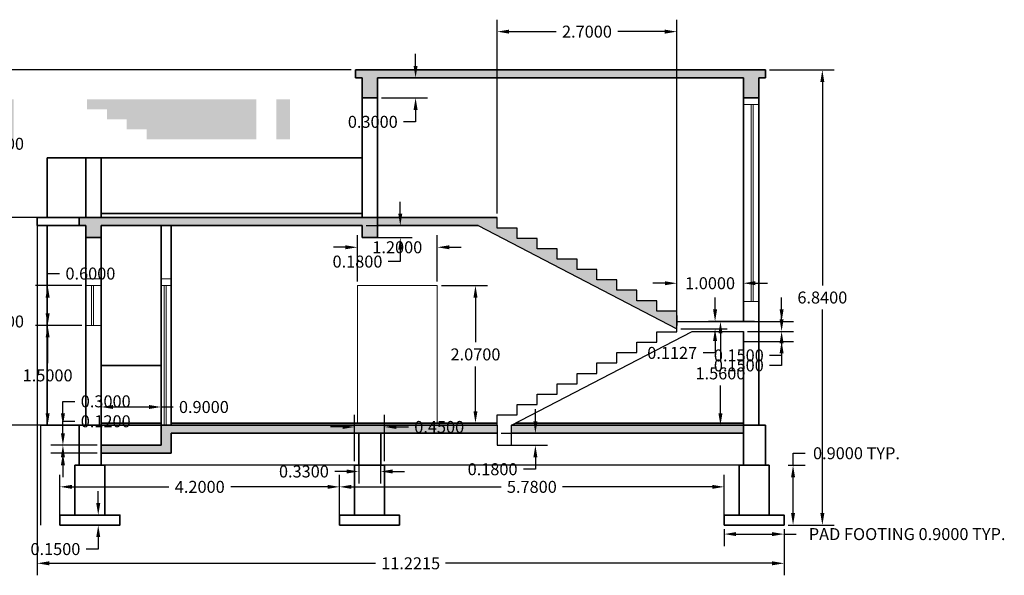
# Model space of a CAD drawing. Units: metres. Extents: x 5.2 to 41.7, y 12.2 to 37.4.
# Tile 6 of 6: x 26.9 to 41.7, y 28.3 to 36.7. Entities that reach past the tile are written whole.
import ezdxf

# ---------------------------------------------------------------- set-up
doc = ezdxf.new("R2010")
doc.units = ezdxf.units.M
doc.header["$MEASUREMENT"] = 0
for name, color, linetype, lineweight in [('A-ANNO-DIMS', 2, 'Continuous', 18), ('A-DOOR', 4, 'Continuous', 18), ('A-FLOR-PLIN', 7, 'Continuous', 25), ('A-FLOR-STRS', 7, 'Continuous', 25), ('A-SECT', 7, 'Continuous', 35), ('S-FNDN', 1, 'Continuous', 35), ('S-SLAB', 7, 'Continuous', 35)]:
    doc.layers.add(name, color=color, linetype=linetype, lineweight=lineweight)
for name, color, linetype, lineweight, true_color in [('A-GLAZ', 51, 'Continuous', 18, 0xf7f281), ('A-PLIN-PATT', 251, 'Continuous', 13, 0x636466), ('S-CONC-PATT', 251, 'Continuous', 13, 0x636466)]:
    doc.layers.add(name, color=color, linetype=linetype, lineweight=lineweight, true_color=true_color)
doc.styles.get("Standard").update_dxf_attribs({"font": 'arial.ttf'})
doc.dimstyles.get("Standard").update_dxf_attribs({"dimtxt": 0.18, "dimasz": 0.18, "dimexe": 0.18, "dimexo": 0.0625, "dimgap": 0.09, "dimtad": 0, "dimtih": 1, "dimtoh": 1, "dimdec": 4, "dimzin": 0, "dimdsep": 46, "dimtxsty": 'Standard', "dimcen": 0.09, "dimadec": 0, "dimazin": 0, "dimtfac": 1, "dimtdec": 4, "dimtofl": 0, "dimtmove": 0, "dimatfit": 3, "dimfxl": 1, "dimtolj": 1, "dimtzin": 0, "dimarcsym": 0})

# ---------------------------------------------------------------- blocks, each defined once
blk = doc.blocks.new('PAD-FOOTING-SECT-900')
for points in [[(0.225, 0.9), (0.675, 0.9), (0.675, 0.15), (0.225, 0.15)], [(0, 0.15), (0.9, 0.15), (0.9, 0), (0, 0)]]:
    blk.add_lwpolyline(points, close=True)
blk = doc.blocks.new('*D24')
at = {"layer": 'A-ANNO-DIMS', "color": 0, "lineweight": -2, "transparency": 16777216}
for p, q in [((37.489, 29.018), (37.489, 28.765)), ((38.389, 29.018), (38.389, 28.765)), ((37.669, 28.945), (38.209, 28.945)), ((38.389, 28.945), (38.569, 28.945))]:
    blk.add_line(p, q, dxfattribs=at)
at = {"layer": 'A-ANNO-DIMS', "color": 0, "lineweight": 25, "transparency": 16777216}
for points in [[(37.669, 28.975), (37.669, 28.915), (37.489, 28.945)], [(38.209, 28.975), (38.209, 28.915), (38.389, 28.945)]]:
    blk.add_solid(points, dxfattribs=at)
at = {"layer": 'Defpoints', "color": 0, "lineweight": 25, "transparency": 16777216}
for p in [(37.489, 29.08), (38.389, 29.08), (38.389, 28.945)]:
    blk.add_point(p, dxfattribs=at)
at = {"layer": 'A-ANNO-DIMS', "color": 0, "transparency": 16777216, "insert": (40.238, 28.945), "char_height": 0.18, "attachment_point": 5}
blk.add_mtext('\\A1;PAD FOOTING 0.9000 TYP.', dxfattribs=at)
blk = doc.blocks.new('*D25')
at = {"layer": 'A-ANNO-DIMS', "color": 0, "lineweight": -2, "transparency": 16777216}
for p, q in [((38.524, 29.98), (38.524, 30.16)), ((38.524, 30.16), (38.704, 30.16)), ((38.452, 29.98), (38.704, 29.98)), ((38.524, 29.26), (38.524, 29.8)), ((38.452, 29.08), (38.704, 29.08))]:
    blk.add_line(p, q, dxfattribs=at)
at = {"layer": 'A-ANNO-DIMS', "color": 0, "lineweight": 25, "transparency": 16777216}
for points in [[(38.494, 29.8), (38.554, 29.8), (38.524, 29.98)], [(38.494, 29.26), (38.554, 29.26), (38.524, 29.08)]]:
    blk.add_solid(points, dxfattribs=at)
at = {"layer": 'Defpoints', "color": 0, "lineweight": 25, "transparency": 16777216}
for p in [(38.389, 29.98), (38.524, 29.98), (38.389, 29.08)]:
    blk.add_point(p, dxfattribs=at)
at = {"layer": 'A-ANNO-DIMS', "color": 0, "transparency": 16777216, "insert": (39.477, 30.16), "char_height": 0.18, "attachment_point": 5}
blk.add_mtext('\\A1;0.9000 TYP.', dxfattribs=at)
blk = doc.blocks.new('*D46')
at = {"layer": 'A-ANNO-DIMS', "color": 0, "lineweight": -2, "transparency": 16777216}
for p, q in [((27.167, 33.638), (27.167, 28.326)), ((38.389, 29.018), (38.389, 28.326)), ((27.347, 28.506), (32.252, 28.506)), ((38.209, 28.506), (33.304, 28.506))]:
    blk.add_line(p, q, dxfattribs=at)
at = {"layer": 'A-ANNO-DIMS', "color": 0, "lineweight": 25, "transparency": 16777216}
for points in [[(27.347, 28.536), (27.347, 28.476), (27.167, 28.506)], [(38.209, 28.536), (38.209, 28.476), (38.389, 28.506)]]:
    blk.add_solid(points, dxfattribs=at)
at = {"layer": 'Defpoints', "color": 0, "lineweight": 25, "transparency": 16777216}
for p in [(27.167, 33.7), (38.389, 29.08), (38.389, 28.506)]:
    blk.add_point(p, dxfattribs=at)
at = {"layer": 'A-ANNO-DIMS', "color": 0, "transparency": 16777216, "insert": (32.778, 28.506), "char_height": 0.18, "attachment_point": 5}
blk.add_mtext('\\A1;11.2215', dxfattribs=at)
blk = doc.blocks.new('*D47')
at = {"layer": 'A-ANNO-DIMS', "color": 0, "lineweight": -2, "transparency": 16777216}
for p, q in [((38.17, 35.92), (39.144, 35.92)), ((38.964, 35.74), (38.964, 32.682)), ((38.964, 29.26), (38.964, 32.318)), ((38.452, 29.08), (39.144, 29.08))]:
    blk.add_line(p, q, dxfattribs=at)
at = {"layer": 'A-ANNO-DIMS', "color": 0, "lineweight": 25, "transparency": 16777216}
for points in [[(38.934, 35.74), (38.994, 35.74), (38.964, 35.92)], [(38.934, 29.26), (38.994, 29.26), (38.964, 29.08)]]:
    blk.add_solid(points, dxfattribs=at)
at = {"layer": 'Defpoints', "color": 0, "lineweight": 25, "transparency": 16777216}
for p in [(38.107, 35.92), (38.964, 35.92), (38.389, 29.08)]:
    blk.add_point(p, dxfattribs=at)
at = {"layer": 'A-ANNO-DIMS', "color": 0, "transparency": 16777216, "insert": (38.964, 32.5), "char_height": 0.18, "attachment_point": 5}
blk.add_mtext('\\A1;6.8400', dxfattribs=at)
blk = doc.blocks.new('*D48')
at = {"layer": 'A-ANNO-DIMS', "color": 0, "lineweight": -2, "transparency": 16777216}
for p, q in [((27.509, 29.143), (27.509, 29.835)), ((31.709, 29.143), (31.709, 29.835)), ((27.689, 29.655), (29.142, 29.655)), ((31.529, 29.655), (30.076, 29.655))]:
    blk.add_line(p, q, dxfattribs=at)
at = {"layer": 'A-ANNO-DIMS', "color": 0, "lineweight": 25, "transparency": 16777216}
for points in [[(27.689, 29.685), (27.689, 29.625), (27.509, 29.655)], [(31.529, 29.685), (31.529, 29.625), (31.709, 29.655)]]:
    blk.add_solid(points, dxfattribs=at)
at = {"layer": 'Defpoints', "color": 0, "lineweight": 25, "transparency": 16777216}
for p in [(31.709, 29.655), (27.509, 29.08), (31.709, 29.08)]:
    blk.add_point(p, dxfattribs=at)
at = {"layer": 'A-ANNO-DIMS', "color": 0, "transparency": 16777216, "insert": (29.609, 29.655), "char_height": 0.18, "attachment_point": 5}
blk.add_mtext('\\A1;4.2000', dxfattribs=at)
blk = doc.blocks.new('*D49')
at = {"layer": 'A-ANNO-DIMS', "color": 0, "lineweight": -2, "transparency": 16777216}
for p, q in [((31.709, 29.143), (31.709, 29.835)), ((37.489, 29.143), (37.489, 29.835)), ((31.889, 29.655), (34.136, 29.655)), ((37.309, 29.655), (35.062, 29.655))]:
    blk.add_line(p, q, dxfattribs=at)
at = {"layer": 'A-ANNO-DIMS', "color": 0, "lineweight": 25, "transparency": 16777216}
for points in [[(31.889, 29.685), (31.889, 29.625), (31.709, 29.655)], [(37.309, 29.685), (37.309, 29.625), (37.489, 29.655)]]:
    blk.add_solid(points, dxfattribs=at)
at = {"layer": 'Defpoints', "color": 0, "lineweight": 25, "transparency": 16777216}
for p in [(37.489, 29.655), (31.709, 29.08), (37.489, 29.08)]:
    blk.add_point(p, dxfattribs=at)
at = {"layer": 'A-ANNO-DIMS', "color": 0, "transparency": 16777216, "insert": (34.599, 29.655), "char_height": 0.18, "attachment_point": 5}
blk.add_mtext('\\A1;5.7800', dxfattribs=at)
blk = doc.blocks.new('*D50')
at = {"layer": 'A-ANNO-DIMS', "color": 0, "lineweight": -2, "transparency": 16777216}
for p, q in [((28.065, 33.7), (26.413, 33.7)), ((26.593, 33.52), (26.593, 32.322)), ((26.593, 30.76), (26.593, 31.958)), ((28.065, 30.58), (26.413, 30.58))]:
    blk.add_line(p, q, dxfattribs=at)
at = {"layer": 'A-ANNO-DIMS', "color": 0, "lineweight": 25, "transparency": 16777216}
for points in [[(26.563, 33.52), (26.623, 33.52), (26.593, 33.7)], [(26.563, 30.76), (26.623, 30.76), (26.593, 30.58)]]:
    blk.add_solid(points, dxfattribs=at)
at = {"layer": 'Defpoints', "color": 0, "lineweight": 25, "transparency": 16777216}
for p in [(26.593, 33.7), (28.127, 33.7), (28.127, 30.58)]:
    blk.add_point(p, dxfattribs=at)
at = {"layer": 'A-ANNO-DIMS', "color": 0, "transparency": 16777216, "insert": (26.593, 32.14), "char_height": 0.18, "attachment_point": 5}
blk.add_mtext('\\A1;3.1200', dxfattribs=at)
blk = doc.blocks.new('*D51')
at = {"layer": 'A-ANNO-DIMS', "color": 0, "lineweight": -2, "transparency": 16777216}
for p, q in [((37.945, 32.14), (37.253, 32.14)), ((37.433, 31.96), (37.433, 31.542)), ((37.433, 30.76), (37.433, 31.178)), ((37.945, 30.58), (37.253, 30.58))]:
    blk.add_line(p, q, dxfattribs=at)
at = {"layer": 'A-ANNO-DIMS', "color": 0, "lineweight": 25, "transparency": 16777216}
for points in [[(37.403, 31.96), (37.463, 31.96), (37.433, 32.14)], [(37.403, 30.76), (37.463, 30.76), (37.433, 30.58)]]:
    blk.add_solid(points, dxfattribs=at)
at = {"layer": 'Defpoints', "color": 0, "lineweight": 25, "transparency": 16777216}
for p in [(37.433, 32.14), (38.007, 32.14), (38.007, 30.58)]:
    blk.add_point(p, dxfattribs=at)
at = {"layer": 'A-ANNO-DIMS', "color": 0, "transparency": 16777216, "insert": (37.433, 31.36), "char_height": 0.18, "attachment_point": 5}
blk.add_mtext('\\A1;1.5600', dxfattribs=at)
blk = doc.blocks.new('*D52')
at = {"layer": 'A-ANNO-DIMS', "color": 0, "lineweight": -2, "transparency": 16777216}
for p, q in [((36.777476, 32.202757), (36.777476, 32.894757)), ((37.777476, 32.202757), (37.777476, 32.894757)), ((36.597476, 32.714757), (36.417476, 32.714757)), ((37.957476, 32.714757), (38.137476, 32.714757))]:
    blk.add_line(p, q, dxfattribs=at)
at = {"layer": 'A-ANNO-DIMS', "color": 0, "lineweight": 25, "transparency": 16777216}
for points in [[(36.597476, 32.744757), (36.597476, 32.684757), (36.777476, 32.714757)], [(37.957476, 32.744757), (37.957476, 32.684757), (37.777476, 32.714757)]]:
    blk.add_solid(points, dxfattribs=at)
at = {"layer": 'Defpoints', "color": 0, "lineweight": 25, "transparency": 16777216}
for p in [(37.777476, 32.714757), (36.777476, 32.140257), (37.777476, 32.140257)]:
    blk.add_point(p, dxfattribs=at)
at = {"layer": 'A-ANNO-DIMS', "color": 0, "transparency": 16777216, "insert": (37.277476, 32.714757), "char_height": 0.18, "attachment_point": 5}
blk.add_mtext('\\A1;1.0000', dxfattribs=at)
blk = doc.blocks.new('*D53')
at = {"layer": 'A-ANNO-DIMS', "color": 0, "lineweight": -2, "transparency": 16777216}
for p, q in [((34.077, 33.763), (34.077, 36.675)), ((36.777, 32.203), (36.777, 36.675)), ((34.257, 36.495), (34.963, 36.495)), ((36.597, 36.495), (35.892, 36.495))]:
    blk.add_line(p, q, dxfattribs=at)
at = {"layer": 'A-ANNO-DIMS', "color": 0, "lineweight": 25, "transparency": 16777216}
for points in [[(34.257, 36.525), (34.257, 36.465), (34.077, 36.495)], [(36.597, 36.525), (36.597, 36.465), (36.777, 36.495)]]:
    blk.add_solid(points, dxfattribs=at)
at = {"layer": 'Defpoints', "color": 0, "lineweight": 25, "transparency": 16777216}
for p in [(36.777, 36.495), (34.077, 33.7), (36.777, 32.14)]:
    blk.add_point(p, dxfattribs=at)
at = {"layer": 'A-ANNO-DIMS', "color": 0, "transparency": 16777216, "insert": (35.427, 36.495), "char_height": 0.18, "attachment_point": 5}
blk.add_mtext('\\A1;2.7000', dxfattribs=at)
blk = doc.blocks.new('*D54')
at = {"layer": 'A-ANNO-DIMS', "color": 0, "lineweight": -2, "transparency": 16777216}
for p, q in [((31.977476, 32.742757), (31.977476, 33.434757)), ((33.177476, 32.742757), (33.177476, 33.434757)), ((31.797476, 33.254757), (31.617476, 33.254757)), ((33.357476, 33.254757), (33.537476, 33.254757))]:
    blk.add_line(p, q, dxfattribs=at)
at = {"layer": 'A-ANNO-DIMS', "color": 0, "lineweight": 25, "transparency": 16777216}
for points in [[(31.797476, 33.284757), (31.797476, 33.224757), (31.977476, 33.254757)], [(33.357476, 33.284757), (33.357476, 33.224757), (33.177476, 33.254757)]]:
    blk.add_solid(points, dxfattribs=at)
at = {"layer": 'Defpoints', "color": 0, "lineweight": 25, "transparency": 16777216}
for p in [(33.177476, 33.254757), (31.977476, 32.680257), (33.177476, 32.680257)]:
    blk.add_point(p, dxfattribs=at)
at = {"layer": 'A-ANNO-DIMS', "color": 0, "transparency": 16777216, "insert": (32.577476, 33.254757), "char_height": 0.18, "attachment_point": 5}
blk.add_mtext('\\A1;1.2000', dxfattribs=at)
blk = doc.blocks.new('*D55')
at = {"layer": 'A-ANNO-DIMS', "color": 0, "lineweight": -2, "transparency": 16777216}
for p, q in [((33.24, 32.68), (33.932, 32.68)), ((33.752, 32.5), (33.752, 31.827)), ((33.752, 30.79), (33.752, 31.463)), ((33.24, 30.61), (33.932, 30.61))]:
    blk.add_line(p, q, dxfattribs=at)
at = {"layer": 'A-ANNO-DIMS', "color": 0, "lineweight": 25, "transparency": 16777216}
for points in [[(33.722, 32.5), (33.782, 32.5), (33.752, 32.68)], [(33.722, 30.79), (33.782, 30.79), (33.752, 30.61)]]:
    blk.add_solid(points, dxfattribs=at)
at = {"layer": 'Defpoints', "color": 0, "lineweight": 25, "transparency": 16777216}
for p in [(33.177, 32.68), (33.177, 30.61), (33.752, 30.61)]:
    blk.add_point(p, dxfattribs=at)
at = {"layer": 'A-ANNO-DIMS', "color": 0, "transparency": 16777216, "insert": (33.752, 31.645), "char_height": 0.18, "attachment_point": 5}
blk.add_mtext('\\A1;2.0700', dxfattribs=at)
blk = doc.blocks.new('*D56')
at = {"layer": 'A-ANNO-DIMS', "color": 0, "lineweight": -2, "transparency": 16777216}
for p, q in [((31.885, 35.92), (26.413, 35.92)), ((26.593, 35.74), (26.593, 34.992)), ((26.593, 33.88), (26.593, 34.628)), ((31.985, 33.7), (26.413, 33.7))]:
    blk.add_line(p, q, dxfattribs=at)
at = {"layer": 'A-ANNO-DIMS', "color": 0, "lineweight": 25, "transparency": 16777216}
for points in [[(26.563, 35.74), (26.623, 35.74), (26.593, 35.92)], [(26.563, 33.88), (26.623, 33.88), (26.593, 33.7)]]:
    blk.add_solid(points, dxfattribs=at)
at = {"layer": 'Defpoints', "color": 0, "lineweight": 25, "transparency": 16777216}
for p in [(26.593, 35.92), (31.947, 35.92), (32.047, 33.7)]:
    blk.add_point(p, dxfattribs=at)
at = {"layer": 'A-ANNO-DIMS', "color": 0, "transparency": 16777216, "insert": (26.593, 34.81), "char_height": 0.18, "attachment_point": 5}
blk.add_mtext('\\A1;2.2200', dxfattribs=at)
blk = doc.blocks.new('*D78')
at = {"layer": 'A-ANNO-DIMS', "color": 0, "lineweight": -2, "transparency": 16777216}
for p, q in [((27.835, 32.08), (27.143, 32.08)), ((27.323, 31.9), (27.323, 31.512)), ((27.323, 30.76), (27.323, 31.148)), ((27.835, 30.58), (27.143, 30.58))]:
    blk.add_line(p, q, dxfattribs=at)
at = {"layer": 'A-ANNO-DIMS', "color": 0, "lineweight": 25, "transparency": 16777216}
for points in [[(27.293, 31.9), (27.353, 31.9), (27.323, 32.08)], [(27.293, 30.76), (27.353, 30.76), (27.323, 30.58)]]:
    blk.add_solid(points, dxfattribs=at)
at = {"layer": 'Defpoints', "color": 0, "lineweight": 25, "transparency": 16777216}
for p in [(27.323, 32.08), (27.897, 32.08), (27.897, 30.58)]:
    blk.add_point(p, dxfattribs=at)
at = {"layer": 'A-ANNO-DIMS', "color": 0, "transparency": 16777216, "insert": (27.323, 31.33), "char_height": 0.18, "attachment_point": 5}
blk.add_mtext('\\A1;1.5000', dxfattribs=at)
blk = doc.blocks.new('*D79')
at = {"layer": 'A-ANNO-DIMS', "color": 0, "lineweight": -2, "transparency": 16777216}
for p, q in [((27.323, 32.68), (27.323, 32.86)), ((27.323, 32.86), (27.503, 32.86)), ((27.835, 32.68), (27.143, 32.68)), ((27.323, 32.26), (27.323, 32.5)), ((27.835, 32.08), (27.143, 32.08))]:
    blk.add_line(p, q, dxfattribs=at)
at = {"layer": 'A-ANNO-DIMS', "color": 0, "lineweight": 25, "transparency": 16777216}
for points in [[(27.293, 32.5), (27.353, 32.5), (27.323, 32.68)], [(27.293, 32.26), (27.353, 32.26), (27.323, 32.08)]]:
    blk.add_solid(points, dxfattribs=at)
at = {"layer": 'Defpoints', "color": 0, "lineweight": 25, "transparency": 16777216}
for p in [(27.323, 32.68), (27.897, 32.68), (27.897, 32.08)]:
    blk.add_point(p, dxfattribs=at)
at = {"layer": 'A-ANNO-DIMS', "color": 0, "transparency": 16777216, "insert": (27.966, 32.86), "char_height": 0.18, "attachment_point": 5}
blk.add_mtext('\\A1;0.6000', dxfattribs=at)
blk = doc.blocks.new('*D80')
at = {"layer": 'A-ANNO-DIMS', "color": 0, "lineweight": -2, "transparency": 16777216}
for p, q in [((28.084, 29.41), (28.084, 29.59)), ((27.572, 29.23), (28.264, 29.23)), ((27.572, 29.08), (28.264, 29.08)), ((28.084, 28.9), (28.084, 28.72)), ((28.084, 28.72), (27.904, 28.72))]:
    blk.add_line(p, q, dxfattribs=at)
at = {"layer": 'A-ANNO-DIMS', "color": 0, "lineweight": 25, "transparency": 16777216}
for points in [[(28.054, 29.41), (28.114, 29.41), (28.084, 29.23)], [(28.054, 28.9), (28.114, 28.9), (28.084, 29.08)]]:
    blk.add_solid(points, dxfattribs=at)
at = {"layer": 'Defpoints', "color": 0, "lineweight": 25, "transparency": 16777216}
for p in [(27.509, 29.23), (27.509, 29.08), (28.084, 29.08)]:
    blk.add_point(p, dxfattribs=at)
at = {"layer": 'A-ANNO-DIMS', "color": 0, "transparency": 16777216, "insert": (27.44, 28.72), "char_height": 0.18, "attachment_point": 5}
blk.add_mtext('\\A1;0.1500', dxfattribs=at)
blk = doc.blocks.new('*D81')
at = {"layer": 'A-ANNO-DIMS', "color": 0, "lineweight": -2, "transparency": 16777216}
for p, q in [((31.934, 30.043), (31.934, 30.735)), ((32.384, 30.043), (32.384, 30.735)), ((31.754, 30.555), (31.574, 30.555)), ((32.564, 30.555), (32.744, 30.555))]:
    blk.add_line(p, q, dxfattribs=at)
at = {"layer": 'A-ANNO-DIMS', "color": 0, "lineweight": 25, "transparency": 16777216}
for points in [[(31.754, 30.585), (31.754, 30.525), (31.934, 30.555)], [(32.564, 30.585), (32.564, 30.525), (32.384, 30.555)]]:
    blk.add_solid(points, dxfattribs=at)
at = {"layer": 'Defpoints', "color": 0, "lineweight": 25, "transparency": 16777216}
for p in [(32.384, 30.555), (31.934, 29.98), (32.384, 29.98)]:
    blk.add_point(p, dxfattribs=at)
at = {"layer": 'A-ANNO-DIMS', "color": 0, "transparency": 16777216, "insert": (33.207, 30.555), "char_height": 0.18, "attachment_point": 5}
blk.add_mtext('\\A1;0.4500', dxfattribs=at)
blk = doc.blocks.new('*D82')
at = {"layer": 'A-ANNO-DIMS', "color": 0, "lineweight": -2, "transparency": 16777216}
for p, q in [((31.997, 30.398), (31.997, 29.706)), ((32.327, 30.398), (32.327, 29.706)), ((31.817, 29.886), (31.637, 29.886)), ((32.507, 29.886), (32.687, 29.886))]:
    blk.add_line(p, q, dxfattribs=at)
at = {"layer": 'A-ANNO-DIMS', "color": 0, "lineweight": 25, "transparency": 16777216}
for points in [[(31.817, 29.916), (31.817, 29.856), (31.997, 29.886)], [(32.507, 29.916), (32.507, 29.856), (32.327, 29.886)]]:
    blk.add_solid(points, dxfattribs=at)
at = {"layer": 'Defpoints', "color": 0, "lineweight": 25, "transparency": 16777216}
for p in [(31.997, 30.46), (32.327, 30.46), (31.997, 29.886)]:
    blk.add_point(p, dxfattribs=at)
at = {"layer": 'A-ANNO-DIMS', "color": 0, "transparency": 16777216, "insert": (31.174, 29.886), "char_height": 0.18, "attachment_point": 5}
blk.add_mtext('\\A1;0.3300', dxfattribs=at)
blk = doc.blocks.new('*D83')
at = {"layer": 'A-ANNO-DIMS', "color": 0, "lineweight": -2, "transparency": 16777216}
for p, q in [((28.127, 30.343), (28.127, 31.035)), ((29.027, 30.343), (29.027, 31.035)), ((28.307, 30.855), (28.847, 30.855)), ((29.027, 30.855), (29.207, 30.855))]:
    blk.add_line(p, q, dxfattribs=at)
at = {"layer": 'A-ANNO-DIMS', "color": 0, "lineweight": 25, "transparency": 16777216}
for points in [[(28.307, 30.885), (28.307, 30.825), (28.127, 30.855)], [(28.847, 30.885), (28.847, 30.825), (29.027, 30.855)]]:
    blk.add_solid(points, dxfattribs=at)
at = {"layer": 'Defpoints', "color": 0, "lineweight": 25, "transparency": 16777216}
for p in [(29.027, 30.855), (28.127, 30.28), (29.027, 30.28)]:
    blk.add_point(p, dxfattribs=at)
at = {"layer": 'A-ANNO-DIMS', "color": 0, "transparency": 16777216, "insert": (29.671, 30.855), "char_height": 0.18, "attachment_point": 5}
blk.add_mtext('\\A1;0.9000', dxfattribs=at)
blk = doc.blocks.new('*D84')
at = {"layer": 'A-ANNO-DIMS', "color": 0, "lineweight": -2, "transparency": 16777216}
for p, q in [((27.553, 30.76), (27.553, 30.94)), ((27.553, 30.94), (27.733, 30.94)), ((28.065, 30.58), (27.373, 30.58)), ((28.065, 30.28), (27.373, 30.28)), ((27.553, 30.1), (27.553, 29.92))]:
    blk.add_line(p, q, dxfattribs=at)
at = {"layer": 'A-ANNO-DIMS', "color": 0, "lineweight": 25, "transparency": 16777216}
for points in [[(27.523, 30.76), (27.583, 30.76), (27.553, 30.58)], [(27.523, 30.1), (27.583, 30.1), (27.553, 30.28)]]:
    blk.add_solid(points, dxfattribs=at)
at = {"layer": 'Defpoints', "color": 0, "lineweight": 25, "transparency": 16777216}
for p in [(27.553, 30.58), (28.127, 30.58), (28.127, 30.28)]:
    blk.add_point(p, dxfattribs=at)
at = {"layer": 'A-ANNO-DIMS', "color": 0, "transparency": 16777216, "insert": (28.196, 30.94), "char_height": 0.18, "attachment_point": 5}
blk.add_mtext('\\A1;0.3000', dxfattribs=at)
blk = doc.blocks.new('*D85')
at = {"layer": 'A-ANNO-DIMS', "color": 0, "lineweight": -2, "transparency": 16777216}
for p, q in [((27.553, 30.46), (27.553, 30.64)), ((27.553, 30.64), (27.733, 30.64)), ((28.065, 30.28), (27.373, 30.28)), ((28.065, 30.16), (27.373, 30.16)), ((27.553, 29.98), (27.553, 29.8))]:
    blk.add_line(p, q, dxfattribs=at)
at = {"layer": 'A-ANNO-DIMS', "color": 0, "lineweight": 25, "transparency": 16777216}
for points in [[(27.523, 30.46), (27.583, 30.46), (27.553, 30.28)], [(27.523, 29.98), (27.583, 29.98), (27.553, 30.16)]]:
    blk.add_solid(points, dxfattribs=at)
at = {"layer": 'Defpoints', "color": 0, "lineweight": 25, "transparency": 16777216}
for p in [(27.553, 30.28), (28.127, 30.28), (28.127, 30.16)]:
    blk.add_point(p, dxfattribs=at)
at = {"layer": 'A-ANNO-DIMS', "color": 0, "transparency": 16777216, "insert": (28.196, 30.64), "char_height": 0.18, "attachment_point": 5}
blk.add_mtext('\\A1;0.1200', dxfattribs=at)
blk = doc.blocks.new('*D86')
at = {"layer": 'A-ANNO-DIMS', "color": 0, "lineweight": -2, "transparency": 16777216}
for p, q in [((32.622, 33.76), (32.622, 33.94)), ((32.11, 33.58), (32.802, 33.58)), ((32.11, 33.4), (32.802, 33.4)), ((32.622, 33.22), (32.622, 33.04)), ((32.622, 33.04), (32.442, 33.04))]:
    blk.add_line(p, q, dxfattribs=at)
at = {"layer": 'A-ANNO-DIMS', "color": 0, "lineweight": 25, "transparency": 16777216}
for points in [[(32.592, 33.76), (32.652, 33.76), (32.622, 33.58)], [(32.592, 33.22), (32.652, 33.22), (32.622, 33.4)]]:
    blk.add_solid(points, dxfattribs=at)
at = {"layer": 'Defpoints', "color": 0, "lineweight": 25, "transparency": 16777216}
for p in [(32.047, 33.58), (32.047, 33.4), (32.622, 33.4)]:
    blk.add_point(p, dxfattribs=at)
at = {"layer": 'A-ANNO-DIMS', "color": 0, "transparency": 16777216, "insert": (31.979, 33.04), "char_height": 0.18, "attachment_point": 5}
blk.add_mtext('\\A1;0.1800', dxfattribs=at)
blk = doc.blocks.new('*D87')
at = {"layer": 'A-ANNO-DIMS', "color": 0, "lineweight": -2, "transparency": 16777216}
for p, q in [((32.852, 35.98), (32.852, 36.16)), ((32.34, 35.8), (33.032, 35.8)), ((32.34, 35.5), (33.032, 35.5)), ((32.852, 35.32), (32.852, 35.14)), ((32.852, 35.14), (32.672, 35.14))]:
    blk.add_line(p, q, dxfattribs=at)
at = {"layer": 'A-ANNO-DIMS', "color": 0, "lineweight": 25, "transparency": 16777216}
for points in [[(32.822, 35.98), (32.882, 35.98), (32.852, 35.8)], [(32.822, 35.32), (32.882, 35.32), (32.852, 35.5)]]:
    blk.add_solid(points, dxfattribs=at)
at = {"layer": 'Defpoints', "color": 0, "lineweight": 25, "transparency": 16777216}
for p in [(32.277, 35.8), (32.277, 35.5), (32.852, 35.5)]:
    blk.add_point(p, dxfattribs=at)
at = {"layer": 'A-ANNO-DIMS', "color": 0, "transparency": 16777216, "insert": (32.209, 35.14), "char_height": 0.18, "attachment_point": 5}
blk.add_mtext('\\A1;0.3000', dxfattribs=at)
blk = doc.blocks.new('*D88')
at = {"layer": 'A-ANNO-DIMS', "color": 0, "lineweight": -2, "transparency": 16777216}
for p, q in [((38.352, 32.17), (38.352, 32.35)), ((37.84, 31.99), (38.532, 31.99)), ((37.84, 31.84), (38.532, 31.84)), ((38.352, 31.66), (38.352, 31.48)), ((38.352, 31.48), (38.172, 31.48))]:
    blk.add_line(p, q, dxfattribs=at)
at = {"layer": 'A-ANNO-DIMS', "color": 0, "lineweight": 25, "transparency": 16777216}
for points in [[(38.322, 32.17), (38.382, 32.17), (38.352, 31.99)], [(38.322, 31.66), (38.382, 31.66), (38.352, 31.84)]]:
    blk.add_solid(points, dxfattribs=at)
at = {"layer": 'Defpoints', "color": 0, "lineweight": 25, "transparency": 16777216}
for p in [(37.777, 31.99), (37.777, 31.84), (38.352, 31.84)]:
    blk.add_point(p, dxfattribs=at)
at = {"layer": 'A-ANNO-DIMS', "color": 0, "transparency": 16777216, "insert": (37.709, 31.48), "char_height": 0.18, "attachment_point": 5}
blk.add_mtext('\\A1;0.1500', dxfattribs=at)
blk = doc.blocks.new('*D89')
at = {"layer": 'A-ANNO-DIMS', "color": 0, "lineweight": -2, "transparency": 16777216}
for p, q in [((38.352, 32.32), (38.352, 32.5)), ((37.84, 32.14), (38.532, 32.14)), ((37.84, 31.99), (38.532, 31.99)), ((38.352, 31.81), (38.352, 31.63)), ((38.352, 31.63), (38.172, 31.63))]:
    blk.add_line(p, q, dxfattribs=at)
at = {"layer": 'A-ANNO-DIMS', "color": 0, "lineweight": 25, "transparency": 16777216}
for points in [[(38.322, 32.32), (38.382, 32.32), (38.352, 32.14)], [(38.322, 31.81), (38.382, 31.81), (38.352, 31.99)]]:
    blk.add_solid(points, dxfattribs=at)
at = {"layer": 'Defpoints', "color": 0, "lineweight": 25, "transparency": 16777216}
for p in [(37.777, 32.14), (37.777, 31.99), (38.352, 31.99)]:
    blk.add_point(p, dxfattribs=at)
at = {"layer": 'A-ANNO-DIMS', "color": 0, "transparency": 16777216, "insert": (37.709, 31.63), "char_height": 0.18, "attachment_point": 5}
blk.add_mtext('\\A1;0.1500', dxfattribs=at)
blk = doc.blocks.new('*D90')
at = {"layer": 'A-ANNO-DIMS', "color": 0, "lineweight": -2, "transparency": 16777216}
for p, q in [((37.352, 32.32), (37.352, 32.5)), ((36.84, 32.14), (37.532, 32.14)), ((36.84, 32.028), (37.532, 32.028)), ((37.352, 31.848), (37.352, 31.668)), ((37.352, 31.668), (37.172, 31.668))]:
    blk.add_line(p, q, dxfattribs=at)
at = {"layer": 'A-ANNO-DIMS', "color": 0, "lineweight": 25, "transparency": 16777216}
for points in [[(37.322, 32.32), (37.382, 32.32), (37.352, 32.14)], [(37.322, 31.848), (37.382, 31.848), (37.352, 32.028)]]:
    blk.add_solid(points, dxfattribs=at)
at = {"layer": 'Defpoints', "color": 0, "lineweight": 25, "transparency": 16777216}
for p in [(36.777, 32.14), (36.777, 32.028), (37.352, 32.028)]:
    blk.add_point(p, dxfattribs=at)
at = {"layer": 'A-ANNO-DIMS', "color": 0, "transparency": 16777216, "insert": (36.708, 31.668), "char_height": 0.18, "attachment_point": 5}
blk.add_mtext('\\A1;0.1127', dxfattribs=at)
blk = doc.blocks.new('*D91')
at = {"layer": 'A-ANNO-DIMS', "color": 0, "lineweight": -2, "transparency": 16777216}
for p, q in [((34.652, 30.64), (34.652, 30.82)), ((34.14, 30.46), (34.832, 30.46)), ((34.14, 30.28), (34.832, 30.28)), ((34.652, 30.1), (34.652, 29.92)), ((34.652, 29.92), (34.472, 29.92))]:
    blk.add_line(p, q, dxfattribs=at)
at = {"layer": 'A-ANNO-DIMS', "color": 0, "lineweight": 25, "transparency": 16777216}
for points in [[(34.622, 30.64), (34.682, 30.64), (34.652, 30.46)], [(34.622, 30.1), (34.682, 30.1), (34.652, 30.28)]]:
    blk.add_solid(points, dxfattribs=at)
at = {"layer": 'Defpoints', "color": 0, "lineweight": 25, "transparency": 16777216}
for p in [(34.077, 30.46), (34.077, 30.28), (34.652, 30.28)]:
    blk.add_point(p, dxfattribs=at)
at = {"layer": 'A-ANNO-DIMS', "color": 0, "transparency": 16777216, "insert": (34.009, 29.92), "char_height": 0.18, "attachment_point": 5}
blk.add_mtext('\\A1;0.1800', dxfattribs=at)

msp = doc.modelspace()

# ---------------------------------------------------------------- hatches: boundary and pattern name
at = {"layer": 'A-PLIN-PATT'}
h = msp.add_hatch(dxfattribs=at)
h.set_pattern_fill('GRAVEL', color=256, scale=0.02)
h.set_pattern_definition([(228.0127875, (0.0144, 0.02), (-0.16, -0.18), [0.00269072, -0.266381761]), (184.9697407, (0.0126, 0.018), (0.24, 0.02), [0.00461736, -0.457118495]), (132.510447, (0.008, 0.0176), (0.2, -0.22), [0.00325576, -0.322320652]), (267.273689, (0.0002, 0.0126), (0.02, 0.4), [0.00420476, -0.416271161]), (292.8336542, (0, 0.0084), (-0.1, 0.24), [0.0041231, -0.4081874626]), (357.273689, (0.0016, 0.0046), (-0.4, 0.02), [0.00420476, -0.416271161]), (37.6942405, (0.0058, 0.0044), (-0.26, -0.2), [0.00556058, -0.550496971]), (72.2553284, (0.0102, 0.0078), (0.14, 0.44), [0.00524976, -0.51972643]), (121.4295656, (0.0118, 0.0128), (-0.16, 0.26), [0.004219, -0.417681462]), (175.2363583, (0.0096, 0.0164), (0.22, -0.02), [0.00481664, -0.2360152516]), (222.3974378, (0.0048, 0.0168), (-0.24, -0.22), [0.00622896, -0.6166675]), (138.814075, (0.02, 0.0124), (-0.14, 0.12), [0.00212602, -0.210476896]), (171.4692344, (0.0184, 0.0138), (0.26, -0.04), [0.00404474, -0.400430228]), (225, (0.0144, 0.0144), (0, -0.02), [0.00282842, -0.025455851]), (203.1985905, (0.013, 0.0168), (0.1, 0.04), [0.00152316, -0.150792302]), (291.8014095, (0.0116, 0.0162), (-0.02, 0.06), [0.00215406, -0.105549236]), (30.9637565, (0.0124, 0.0142), (0.06, 0.04), [0.00349858, -0.113120458]), (161.565051, (0.0154, 0.016), (0.04, -0.02), [0.00252982, -0.060715733]), (16.3895403, (0, 0.0162), (0.2, 0.06), [0.003544, -0.350856903]), (70.346176, (0.0034, 0.0172), (-0.08, -0.22), [0.00297322, -0.294348155]), (293.1985905, (0.0154, 0.02), (-0.04, 0.1), [0.0030463, -0.149269162]), (343.6104597, (0.0166, 0.0172), (-0.2, 0.06), [0.003544, -0.350856903]), (339.443955, (0, 0.0038), (-0.1, 0.04), [0.0034176, -0.167462475]), (294.7751406, (0.0032, 0.0026), (-0.1, 0.22), [0.00286356, -0.283492861]), (66.8014095, (0.0156, 0), (0.04, 0.1), [0.0030463, -0.149269162]), (17.3540246, (0.0168, 0.0028), (-0.26, -0.08), [0.00335262, -0.331908472]), (69.443955, (0.0058, 0), (-0.04, -0.1), [0.0017088, -0.169171275]), (101.309932, (0.0144, 0), (-0.02, 0.08), [0.0010198, -0.10096059]), (165.963757, (0.0142, 0.001), (0.06, -0.02), [0.0041231, -0.0783390125]), (186.009006, (0.0102, 0.002), (0.2, 0.02), [0.003821, -0.3782784635]), (303.690068, (0.0124, 0.0124), (-0.02, 0.04), [0.00288444, -0.0692265855]), (353.1572266, (0.014, 0.01), (0.34, -0.04), [0.00503588, -0.4985512525]), (60.945396, (0.019, 0.0094), (-0.08, -0.14), [0.00205912, -0.203853483]), (90, (0.02, 0.0112), (-0.02, 0.02), [0.0012, -0.0188]), (120.256437, (0.0098, 0.0026), (0.08, -0.14), [0.00277848, -0.2750704]), (48.0127875, (0.0084, 0.005), (0.16, 0.18), [0.00538144, -0.263691041]), (0, (0.012, 0.009), (0.02, 0.02), [0.0052, -0.0148]), (325.3048465, (0.0172, 0.009), (0.2, -0.14), [0.00316228, -0.313065486]), (254.054604, (0.0198, 0.0072), (-0.02, -0.08), [0.00291204, -0.142690158]), (207.6459754, (0.019, 0.0044), (-0.38, -0.2), [0.0047413, -0.469389484]), (175.4260787, (0.0148, 0.0022), (-0.26, 0.02), [0.00501598, -0.496581468])])
h.paths.add_polyline_path([(23.80317, 35.47718), (20.65317, 35.47718), (20.65317, 34.87718), (23.80317, 34.87718)])
h.paths.add_polyline_path([(26.81317, 35.47718), (26.71317, 35.47718), (23.80317, 35.47718), (23.80317, 34.87718), (26.81317, 34.87718)])
h.paths.add_polyline_path([(30.46113, 35.47718), (27.91317, 35.47718), (27.91317, 35.32718), (28.21317, 35.32718), (28.21317, 35.17718), (28.51317, 35.17718), (28.51317, 35.02718), (28.81317, 35.02718), (28.81317, 34.87718), (30.46113, 34.87718)])
h.paths.add_polyline_path([(30.96317, 35.47718), (30.76113, 35.47718), (30.76113, 34.87718), (30.96317, 34.87718)])
at = {"layer": 'S-CONC-PATT'}
h = msp.add_hatch(dxfattribs=at)
h.set_pattern_fill('AR-CONC', color=256, scale=0.01)
h.set_pattern_definition([(50, (-29.48366, -4.896924), (0.07172602, -0.006275213), [0.0075, -0.0825]), (355, (-29.48366, -4.896924), (-0.01387513, 0.07521921), [0.006, -0.066]), (100.45144, (-29.477686, -4.89745), (0.057850885, 0.068944), [0.00637402, -0.07011421]), (46.1842, (-29.48366, -4.876924), (0.10672413, -0.01655193), [0.01125, -0.12375]), (96.63564, (-29.47477, -4.8783), (0.0934662, 0.09741186), [0.00956103, -0.10517138]), (351.18416, (-29.48366, -4.87692), (0.0934662, 0.09741186), [0.009, -0.099]), (21, (-29.47366, -4.881924), (0.059690705, -0.04026189), [0.0075, -0.0825]), (326, (-29.47366, -4.881924), (0.02433153, 0.072515005), [0.006, -0.066]), (71.45144, (-29.46869, -4.88528), (0.08402224, 0.032253115), [0.00637402, -0.07011421]), (37.5, (-29.483663, -4.896924), (0.0012159855, 0.033289385), [0, -0.0652, 0, -0.067, 0, -0.06625]), (7.5, (-29.483663, -4.896924), (0.026306954, 0.039441171), [0, -0.0382, 0, -0.0637, 0, -0.02525]), (327.5, (-29.505963, -4.896924), (0.053382244, -0.002255487), [0, -0.025, 0, -0.078, 0, -0.1035]), (317.5, (-29.515963, -4.896924), (0.058318617, 0.010010498), [0, -0.0325, 0, -0.0518, 0, -0.0735])])
h.paths.add_polyline_path([(32.27748, 33.70026), (27.79748, 33.70026), (27.79748, 33.58026), (27.89748, 33.58026), (27.89748, 33.40026), (28.12748, 33.40026), (28.12748, 33.58026), (32.04748, 33.58026), (32.04748, 33.40026), (32.27748, 33.40026)])
h.paths.add_polyline_path([(29.17748, 30.46026), (34.07748, 30.46026), (34.07748, 30.58026), (29.02748, 30.58026), (29.02748, 30.28026), (28.12748, 30.28026), (28.12748, 30.16026), (29.17748, 30.16026)])
h.paths.add_polyline_path([(37.77748, 30.58026), (34.29423, 30.58026), (34.29423, 30.46026), (37.77748, 30.46026)])
h.paths.add_polyline_path([(34.07748, 33.70026), (33.77748, 33.70026), (32.27748, 33.70026), (32.27748, 33.58026), (33.79149, 33.58026), (36.77748, 32.02754), (36.77748, 32.14026), (36.77748, 32.29626), (36.47748, 32.29626), (36.47748, 32.45226), (36.17748, 32.45226), (36.17748, 32.60826), (35.87748, 32.60826), (35.87748, 32.76426), (35.57748, 32.76426), (35.57748, 32.92026), (35.27748, 32.92026), (35.27748, 33.07626), (34.97748, 33.07626), (34.97748, 33.23226), (34.67748, 33.23226), (34.67748, 33.38826), (34.37748, 33.38826), (34.37748, 33.54426), (34.07748, 33.54426)])
h.paths.add_polyline_path([(38.10748, 35.92026), (31.94748, 35.92026), (31.94748, 35.80026), (32.04748, 35.80026), (32.04748, 35.50026), (32.27748, 35.50026), (32.27748, 35.80026), (37.77748, 35.80026), (37.77748, 35.50026), (38.00748, 35.50026), (38.00748, 35.80026), (38.10748, 35.80026)])

# ---------------------------------------------------------------- linework, layer by layer
at = {"layer": 'A-DOOR'}
for p, q in [((29.02748, 32.78026), (29.17748, 32.78026)), ((29.02748, 32.68026), (29.17748, 32.68026)), ((29.07248, 32.68026), (29.07248, 30.58026)), ((29.10248, 32.68026), (29.10248, 30.58026))]:
    msp.add_line(p, q, dxfattribs=at)
for points in [[(31.97748, 30.61026), (31.97748, 32.68026), (33.17748, 32.68026), (33.17748, 30.61026)], [(33.17748, 30.58026), (31.97748, 30.58026)]]:
    msp.add_lwpolyline(points, dxfattribs=at)
at = {"layer": 'A-FLOR-PLIN'}
for p, q in [((27.21748, 30.58026), (27.21748, 29.08026)), ((27.79748, 29.98026), (27.79748, 30.58026)), ((38.10748, 30.58026), (38.10748, 29.98026)), ((38.10748, 29.98026), (27.79748, 29.98026))]:
    msp.add_line(p, q, dxfattribs=at)
at = {"layer": 'A-FLOR-STRS'}
for p, q in [((33.79149, 33.58026), (36.77748, 32.02754)), ((36.77748, 32.23026), (36.77748, 32.08026)), ((34.29423, 30.58026), (37.00577, 31.99026)), ((36.77748, 31.98426), (36.77748, 32.08026)), ((37.00577, 31.99026), (37.77748, 31.99026)), ((34.07748, 30.58026), (34.07748, 30.28026)), ((34.29423, 30.28026), (34.29423, 30.58026)), ((34.07748, 30.28026), (34.29423, 30.28026))]:
    msp.add_line(p, q, dxfattribs=at)
for points in [[(34.07748, 33.54426), (34.07748, 33.70026), (33.77748, 33.70026)], [(34.37748, 33.38826), (34.37748, 33.54426), (34.07748, 33.54426)], [(34.67748, 33.23226), (34.67748, 33.38826), (34.37748, 33.38826)], [(34.97748, 33.07626), (34.97748, 33.23226), (34.67748, 33.23226)], [(35.27748, 32.92026), (35.27748, 33.07626), (34.97748, 33.07626)], [(35.57748, 32.76426), (35.57748, 32.92026), (35.27748, 32.92026)], [(35.87748, 32.60826), (35.87748, 32.76426), (35.57748, 32.76426)], [(36.17748, 32.45226), (36.17748, 32.60826), (35.87748, 32.60826)], [(36.47748, 32.29626), (36.47748, 32.45226), (36.17748, 32.45226)], [(36.47748, 32.29626), (36.47748, 32.44026)], [(36.77748, 32.14026), (36.77748, 32.29626), (36.47748, 32.29626)], [(36.77748, 31.98426), (36.77748, 32.14026), (38.00748, 32.14026)], [(36.47748, 31.82826), (36.47748, 31.98426), (36.77748, 31.98426)], [(36.17748, 31.67226), (36.17748, 31.82826), (36.47748, 31.82826)], [(37.77748, 31.84026), (38.00748, 31.84026)], [(35.87748, 31.51626), (35.87748, 31.67226), (36.17748, 31.67226)], [(35.57748, 31.36026), (35.57748, 31.51626), (35.87748, 31.51626)], [(35.27748, 31.20426), (35.27748, 31.36026), (35.57748, 31.36026)], [(34.97748, 31.04826), (34.97748, 31.20426), (35.27748, 31.20426)], [(34.67748, 30.89226), (34.67748, 31.04826), (34.97748, 31.04826)], [(34.37748, 30.73626), (34.37748, 30.89226), (34.67748, 30.89226)], [(34.07748, 30.58026), (34.07748, 30.73626), (34.37748, 30.73626)]]:
    msp.add_lwpolyline(points, dxfattribs=at)
at = {"layer": 'A-GLAZ'}
for p, q in [((37.89248, 35.40026), (37.89248, 32.44026)), ((37.92248, 35.40026), (37.92248, 32.44026)), ((27.89748, 32.78026), (28.12748, 32.78026)), ((27.89748, 32.68026), (28.12748, 32.68026)), ((27.98248, 32.68026), (27.98248, 32.08026)), ((28.01248, 32.68026), (28.01248, 32.08026)), ((27.89748, 32.08026), (28.12748, 32.08026))]:
    msp.add_line(p, q, dxfattribs=at)
for points in [[(37.77748, 35.40026), (38.00748, 35.40026)], [(37.77748, 32.44026), (38.00748, 32.44026)]]:
    msp.add_lwpolyline(points, dxfattribs=at)
at = {"layer": 'A-SECT'}
for p, q in [((37.77748, 32.14026), (37.77748, 35.80026)), ((38.00748, 35.80026), (38.00748, 30.58026)), ((27.31748, 34.60026), (32.04748, 34.60026)), ((27.31748, 33.70026), (27.31748, 34.60026)), ((27.89748, 33.70026), (27.89748, 34.60026)), ((28.12748, 33.70026), (28.12748, 34.60026)), ((27.31748, 30.58026), (27.31748, 33.58026)), ((27.89748, 30.58026), (27.89748, 33.58026)), ((28.12748, 30.58026), (28.12748, 33.58026)), ((29.02748, 30.28026), (29.02748, 33.58026)), ((29.17748, 33.58026), (29.17748, 30.58026)), ((37.77748, 30.58026), (37.77748, 31.99026)), ((28.12748, 31.48026), (29.02748, 31.48026))]:
    msp.add_line(p, q, dxfattribs=at)
for points in [[(32.04748, 33.70026), (32.04748, 35.80026)], [(32.27748, 35.80026), (32.27748, 33.40026)]]:
    msp.add_lwpolyline(points, dxfattribs=at)
at = {"layer": 'S-FNDN'}
for points in [[(28.12748, 30.58026), (27.79748, 30.58026), (27.79748, 29.98026), (28.12748, 29.98026)], [(38.10748, 30.58026), (37.77748, 30.58026), (37.77748, 29.98026), (38.10748, 29.98026)], [(32.32748, 30.46026), (31.99748, 30.46026), (31.99748, 29.98026), (32.32748, 29.98026)]]:
    msp.add_lwpolyline(points, close=True, dxfattribs=at)
at = {"layer": 'S-SLAB'}
for p, q in [((31.94748, 35.92026), (38.10748, 35.92026)), ((38.10748, 35.92026), (38.10748, 35.80026)), ((31.94748, 35.80026), (32.04748, 35.80026)), ((32.27748, 35.80026), (37.77748, 35.80026)), ((38.00748, 35.80026), (38.10748, 35.80026)), ((32.04748, 35.50026), (32.27748, 35.50026)), ((37.77748, 35.50026), (38.00748, 35.50026)), ((28.12748, 33.76026), (32.04748, 33.76026)), ((27.16748, 33.70026), (32.27748, 33.70026)), ((27.16748, 33.70026), (27.16748, 33.58026)), ((27.79748, 33.58026), (27.79748, 33.70026)), ((32.27748, 33.70026), (34.07748, 33.70026)), ((27.89748, 33.58026), (27.16748, 33.58026)), ((32.04748, 33.58026), (28.12748, 33.58026)), ((33.79149, 33.58026), (32.27748, 33.58026)), ((27.89748, 33.40026), (28.12748, 33.40026)), ((32.04748, 33.40026), (32.27748, 33.40026)), ((27.21748, 30.58026), (34.07748, 30.58026)), ((28.12748, 30.61026), (29.02748, 30.61026)), ((29.17748, 30.61026), (34.07748, 30.61026)), ((34.29423, 30.58026), (38.10748, 30.58026)), ((34.35192, 30.61026), (37.77748, 30.61026)), ((29.17748, 30.46026), (34.07748, 30.46026)), ((29.17748, 30.46026), (29.17748, 30.16026)), ((34.29423, 30.46026), (37.77748, 30.46026)), ((28.12748, 30.28026), (29.02748, 30.28026)), ((28.12748, 30.16026), (29.17748, 30.16026))]:
    msp.add_line(p, q, dxfattribs=at)
for points in [[(31.94748, 35.80026), (31.94748, 35.92026)], [(32.04748, 33.40026), (32.04748, 33.58026)]]:
    msp.add_lwpolyline(points, dxfattribs=at)

# ---------------------------------------------------------------- block references
at = {"layer": 'S-FNDN'}
for p in [(27.509, 29.08), (31.709, 29.08), (37.489, 29.08)]:
    msp.add_blockref('PAD-FOOTING-SECT-900', p, dxfattribs=at)

# ---------------------------------------------------------------- dimensions: what is measured, and where the dimension line sits
at = {"layer": 'A-ANNO-DIMS'}
for base, p1, p2, picture, middle in [((36.77748, 36.49476), (34.07748, 33.70026), (36.77748, 32.14026), '*D53', (35.42748, 36.49476)), ((38.38901, 28.50576), (27.16748, 33.70026), (38.38901, 29.08026), '*D46', (32.77824, 28.50576)), ((33.17748, 33.25476), (31.97748, 32.68026), (33.17748, 32.68026), '*D54', (32.57748, 33.25476)), ((37.77748, 32.71476), (36.77748, 32.14026), (37.77748, 32.14026), '*D52', (37.27748, 32.71476)), ((29.02748, 30.85476), (28.12748, 30.28026), (29.02748, 30.28026), '*D83', (29.6708, 30.85476)), ((32.38401, 30.55476), (31.93401, 29.98026), (32.38401, 29.98026), '*D81', (33.20733, 30.55476)), ((31.70901, 29.65476), (27.50901, 29.08026), (31.70901, 29.08026), '*D48', (29.60901, 29.65476)), ((37.48901, 29.65476), (31.70901, 29.08026), (37.48901, 29.08026), '*D49', (34.59901, 29.65476))]:
    dim = msp.add_linear_dim(base=base, p1=p1, p2=p2, dimstyle='Standard', override={"dimdec": 4, "dimlfac": 1, "dimrnd": 0, "dimzin": 0, "dimdsep": 46, "dimlunit": 2}, dxfattribs=at)
    dim.commit()
    dim.dimension.update_dxf_attribs({"geometry": picture, "text_midpoint": middle})
for base, p1, p2, angle, picture, middle in [((32.85198, 35.50026), (32.27748, 35.80026), (32.27748, 35.50026), 270, '*D87', (32.20865, 35.14026)), ((26.59298, 35.92026), (32.04748, 33.70026), (31.94748, 35.92026), 90, '*D56', (26.59298, 34.81026)), ((38.96351, 35.92026), (38.38901, 29.08026), (38.10748, 35.92026), 90, '*D47', (38.96351, 32.50026)), ((32.62198, 33.40026), (32.04748, 33.58026), (32.04748, 33.40026), 270, '*D86', (31.97865, 33.04026)), ((26.59298, 33.70026), (28.12748, 30.58026), (28.12748, 33.70026), 90, '*D50', (26.59298, 32.14026)), ((27.32298, 32.68026), (27.89748, 32.08026), (27.89748, 32.68026), 90, '*D79', (27.9663, 32.86026)), ((33.75198, 30.61026), (33.17748, 32.68026), (33.17748, 30.61026), 270, '*D55', (33.75198, 31.64526)), ((37.35198, 32.02755), (36.77748, 32.14026), (36.77748, 32.02755), 270, '*D90', (36.70835, 31.66755)), ((38.35198, 31.99026), (37.77748, 32.14026), (37.77748, 31.99026), 270, '*D89', (37.70865, 31.63026)), ((38.35198, 31.84026), (37.77748, 31.99026), (37.77748, 31.84026), 270, '*D88', (37.70865, 31.48026)), ((37.43298, 32.14026), (38.00748, 30.58026), (38.00748, 32.14026), 90, '*D51', (37.43298, 31.36026)), ((27.32298, 32.08026), (27.89748, 30.58026), (27.89748, 32.08026), 90, '*D78', (27.32298, 31.33026)), ((27.55298, 30.58026), (28.12748, 30.28026), (28.12748, 30.58026), 90, '*D84', (28.1963, 30.94026)), ((34.65198, 30.28026), (34.07748, 30.46026), (34.07748, 30.28026), 270, '*D91', (34.00865, 29.92026)), ((27.55298, 30.28026), (28.12748, 30.16026), (28.12748, 30.28026), 90, '*D85', (28.1963, 30.64026)), ((31.99748, 29.88576), (32.32748, 30.46026), (31.99748, 30.46026), 180, '*D82', (31.17415, 29.88576)), ((28.08351, 29.08026), (27.50901, 29.23026), (27.50901, 29.08026), 270, '*D80', (27.44019, 28.72026))]:
    dim = msp.add_linear_dim(base=base, p1=p1, p2=p2, angle=angle, dimstyle='Standard', override={"dimdec": 4, "dimlfac": 1, "dimrnd": 0, "dimzin": 0, "dimdsep": 46, "dimlunit": 2}, dxfattribs=at)
    dim.commit()
    dim.dimension.update_dxf_attribs({"geometry": picture, "text_midpoint": middle})
dim = msp.add_linear_dim(base=(38.52401, 29.98026), p1=(38.38901, 29.08026), p2=(38.38901, 29.98026), angle=90, text='<> TYP.', dimstyle='Standard', override={"dimdec": 4, "dimlfac": 1, "dimrnd": 0, "dimzin": 0, "dimdsep": 46, "dimlunit": 2}, dxfattribs=at)
dim.commit()
dim.dimension.update_dxf_attribs({"geometry": '*D25', "text_midpoint": (39.47681, 30.16026)})
dim = msp.add_linear_dim(base=(38.38901, 28.94526), p1=(37.48901, 29.08026), p2=(38.38901, 29.08026), text='PAD FOOTING <> TYP.', dimstyle='Standard', override={"dimdec": 4, "dimlfac": 1, "dimrnd": 0, "dimzin": 0, "dimdsep": 46, "dimlunit": 2}, dxfattribs=at)
dim.commit()
dim.dimension.update_dxf_attribs({"geometry": '*D24', "text_midpoint": (40.23843, 28.94526)})

doc.saveas('drawing.dxf')
